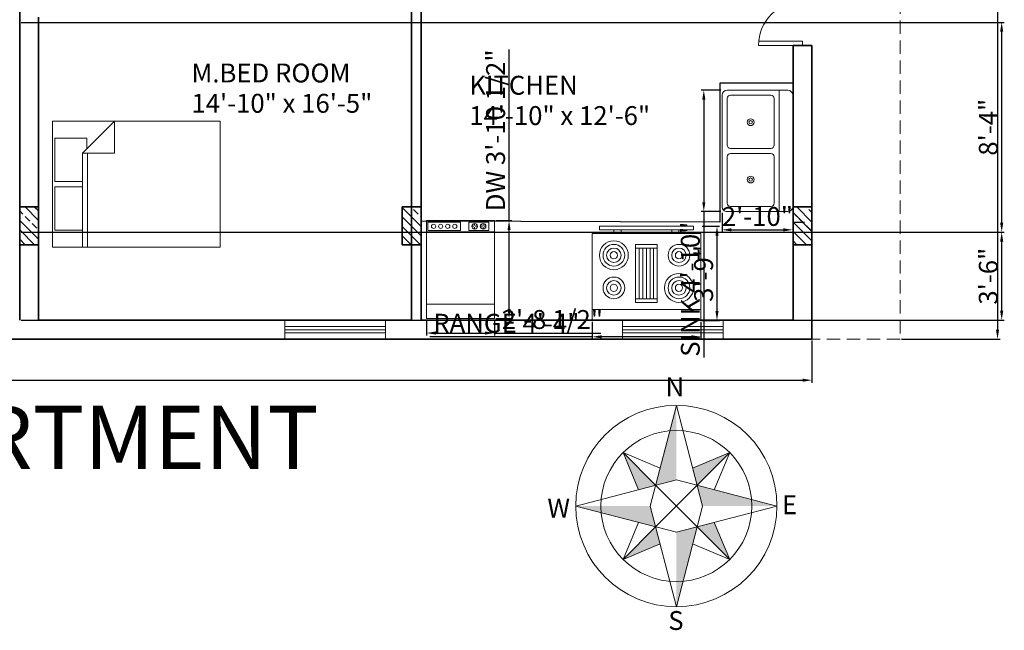
# Model space of a CAD drawing. Units: inches. Extents: x 2081 to 4786, y 1256 to 3802.
# Tile 6 of 7: x 2685 to 3155, y 1294 to 1585. Entities that reach past the tile are written whole.
import ezdxf

# ---------------------------------------------------------------- set-up
doc = ezdxf.new("R2010")
doc.units = ezdxf.units.IN
doc.linetypes.add('HIDDEN', pattern=[9.525, 6.35, -3.175])
for name, color, linetype, lineweight in [('A-ANNO-DIMS', 18, 'Continuous', 18), ('A-ANNO-SYMB', 18, 'Continuous', 18), ('A-ANNO-TITL', 18, 'Continuous', 35), ('A-AREA-IDEN', 18, 'Continuous', 18), ('A-COLS', 1, 'Continuous', 35), ('A-DOOR', 5, 'Continuous', 18), ('A-EQPM', 11, 'Continuous', 18), ('A-FLOR-CASE', 7, 'Continuous', 25), ('A-FLOR-FIXT', 18, 'Continuous', 18), ('A-FLOR-OVHD', 18, 'HIDDEN', 18), ('A-FURN', 5, 'Continuous', 18), ('A-GLAZ', 11, 'Continuous', 18), ('A-WALL', 7, 'Continuous', 35)]:
    doc.layers.add(name, color=color, linetype=linetype, lineweight=lineweight)
doc.styles.get("Standard").update_dxf_attribs({"font": 'arial.ttf'})
doc.dimstyles.new('ISO-25', dxfattribs={"dimtxt": 9, "dimasz": 4.5, "dimexe": 1.25, "dimexo": 0.625, "dimtad": 1, "dimdec": 0, "dimlunit": 3, "dimtxsty": 'Standard', "dimcen": 2.5, "dimadec": 0, "dimazin": 0, "dimtfac": 1, "dimtdec": 0, "dimtmove": 0, "dimatfit": 3, "dimfxl": 1, "dimarcsym": 0})
pattern_1 = [(135, (1916.44, -3174.735), (-13.47038, -13.47038), []), (135, (1916.44, -3170.245), (-13.47038, -13.47038), []), (135, (1916.44, -3165.755), (-13.47038, -13.47038), []), (135, (1916.44, -3161.265), (-13.47038, -13.47038), [])]

# ---------------------------------------------------------------- blocks, each defined once
blk = doc.blocks.new('Bed - Queen')
for p, q in [((0, -80.00003), (0, 0)), ((0, 0), (59.99999, 0)), ((59.99999, 0), (59.99999, -80.00003)), ((7.99999, -1.2), (28.79998, -1.2)), ((7.99999, -14.4), (7.99999, -1.2)), ((28.79998, -1.2), (28.79998, -14.4)), ((31.19999, -1.2), (51.99999, -1.2)), ((31.19999, -14.4), (31.19999, -1.2)), ((51.99999, -1.2), (51.99999, -16.4)), ((0, -14.4), (44.8, -14.4)), ((44.8, -16.8), (0, -16.8)), ((59.99999, -29.6), (44.8, -14.4)), ((44.8, -14.4), (44.8, -29.6)), ((51.99999, -16.4), (46.79936, -16.4)), ((44.8, -29.6), (59.99999, -29.6)), ((59.99999, -80.00003), (0, -80.00003))]:
    blk.add_line(p, q)
blk = doc.blocks.new('Range-Oven - 30 in top')
for p, q in [((0, -3), (30, -3)), ((12, -6), (18, -6)), ((13, -20), (13, -6)), ((14, -6), (14, -20)), ((15, -20), (15, -6)), ((16, -6), (16, -20)), ((17, -20), (17, -6)), ((18, -20), (12, -20)), ((6, -24), (6, -25)), ((8, -25), (8, -24)), ((22, -25), (22, -24)), ((24, -24), (24, -25))]:
    blk.add_line(p, q)
for points in [[(0, -24), (0, 0), (30, 0), (30, -24)], [(12, -21), (12, -5), (18, -5), (18, -21)], [(2, -26), (2, -25), (28, -25), (28, -26)]]:
    blk.add_lwpolyline(points, close=True)
for centre, radius in [((6, -9), 4), ((6, -9), 3), ((6, -9), 2), ((6, -9), 1), ((24, -9), 3), ((24, -9), 2), ((24, -9), 1), ((6, -18), 3), ((6, -18), 2), ((24, -18), 4), ((24, -18), 3), ((24, -18), 2), ((6, -18), 1), ((24, -18), 1)]:
    blk.add_circle(centre, radius)
blk = doc.blocks.new('Dishwasher')
for p, q in [((16, 32.5), (16.75, 32.5)), ((16.5, 32), (16.2942, 31.7942)), ((16.3156, 33.1843), (16.5, 33)), ((17, 32.75), (17, 33.5)), ((17, 32.25), (17, 31.5)), ((18, 32.5), (17.25, 32.5)), ((17.5, 33), (17.6938, 33.1938)), ((17.7061, 31.7939), (17.5, 32)), ((19, 32.5), (19.75, 32.5)), ((19.5, 32), (19.2942, 31.7942)), ((19.3156, 33.1843), (19.5, 33)), ((20, 32.75), (20, 33.5)), ((20, 32.25), (20, 31.5)), ((21, 32.5), (20.25, 32.5)), ((20.5, 33), (20.6938, 33.1938)), ((20.7061, 31.7939), (20.5, 32)), ((24, 30.5), (0, 30.5)), ((0, 5), (24, 5))]:
    blk.add_line(p, q)
for points in [[(0, 0), (0, 34.5), (24, 34.5), (24, 0)], [(0.5, 31), (0.5, 34), (12, 34), (12, 31)], [(15, 31), (15, 34), (22, 34), (22, 31)]]:
    blk.add_lwpolyline(points, close=True)
for centre, radius in [((2.5, 32.5), 0.75), ((5, 32.5), 0.75), ((7.5, 32.5), 0.75), ((10, 32.5), 0.75), ((17, 32.5), 1), ((20, 32.5), 1)]:
    blk.add_circle(centre, radius)
blk = doc.blocks.new('Sink-double - 36 in top')
for p, q in [((-18, -4), (18, -4)), ((-0.75, -18.5), (-0.75, -6.5)), ((0.75, -6.5), (0.75, -18.5))]:
    blk.add_line(p, q)
for points in [[(-16.5, 0), (16.5, 0)], [(-18, -19.5), (-18, -1.5)], [(18, -1.5), (18, -19.5)], [(-15.5, -5.5), (-1.75, -5.5)], [(1.75, -5.5), (15.5, -5.5)], [(-16.5, -18.5), (-16.5, -6.5)], [(16.5, -6.5), (16.5, -18.5)], [(-1.75, -19.5), (-15.5, -19.5)], [(15.5, -19.5), (1.75, -19.5)], [(16.5, -21), (-16.5, -21)]]:
    blk.add_lwpolyline(points)
for centre, radius in [((-8.5, -12.5), 1), ((8.5, -12.5), 1), ((-8.5, -12.5), 0.5), ((8.5, -12.5), 0.5)]:
    blk.add_circle(centre, radius)
for centre, radius, start, end in [((-16.5, -1.5), 1.5, 90, 180), ((16.5, -1.5), 1.5, 0, 90), ((-15.5, -6.5), 1, 90, 180), ((-1.75, -6.5), 1, 0, 90), ((1.75, -6.5), 1, 90, 180), ((15.5, -6.5), 1, 0, 90), ((-16.5, -19.5), 1.5, 180, 270), ((-15.5, -18.5), 1, 180, 270), ((-1.75, -18.5), 1, 270, 0), ((1.75, -18.5), 1, 180, 270), ((15.5, -18.5), 1, 270, 0), ((16.5, -19.5), 1.5, 270, 0)]:
    blk.add_arc(centre, radius, start, end)
blk = doc.blocks.new('*U19')
for q in [(-12.45, -24), (12.45, -24)]:
    blk.add_line((0, 24), q)
blk = doc.blocks.new('*U20')
at = {"layer": 'A-ANNO-SYMB', "color": 0, "linetype": 'ByBlock', "lineweight": -2, "transparency": 16777216}
blk.add_blockref('*U19', (2998.28, 1377.6), dxfattribs=at)
for p, rotation in [((2974.28, 1353.6), 90), ((3022.28, 1353.6), 270), ((2998.28, 1329.6), 180)]:
    blk.add_blockref('*U19', p, dxfattribs=dict(at, rotation=rotation))
blk = doc.blocks.new('*U21')
for q in [(-8.84, 1.4), (1.4, -8.84)]:
    blk.add_line((8.84, 8.84), q)
blk = doc.blocks.new('*U22')
at = {"layer": 'A-ANNO-SYMB', "color": 0, "linetype": 'ByBlock', "lineweight": -2, "transparency": 16777216}
for p, rotation in [((2981.66, 1370.22), 90.00000000000003), ((2981.66, 1336.98), 180), ((3014.89, 1336.98), 270)]:
    blk.add_blockref('*U21', p, dxfattribs=dict(at, rotation=rotation))
blk.add_blockref('*U21', (3014.89, 1370.22), dxfattribs=at)
blk = doc.blocks.new('*D24')
at = {"layer": 'A-ANNO-DIMS', "color": 0, "lineweight": -2, "transparency": 16777216}
for p, q in [((3105.61, 2023.17), (3152.75, 2023.17)), ((3151.5, 2018.67), (3151.5, 1437.67)), ((3105.61, 1433.17), (3152.75, 1433.17))]:
    blk.add_line(p, q, dxfattribs=at)
at = {"layer": 'A-ANNO-DIMS', "color": 0, "transparency": 16777216}
for points in [[(3150.75, 2018.67), (3152.25, 2018.67), (3151.5, 2023.17)], [(3150.75, 1437.67), (3152.25, 1437.67), (3151.5, 1433.17)]]:
    blk.add_solid(points, dxfattribs=at)
at = {"layer": 'Defpoints', "color": 0, "transparency": 16777216}
for p in [(3104.98, 2023.17), (3104.98, 1433.17), (3151.5, 1433.17)]:
    blk.add_point(p, dxfattribs=at)
at = {"layer": 'A-ANNO-DIMS', "color": 0, "transparency": 16777216, "insert": (3146.28, 1728.17), "char_height": 9, "attachment_point": 5, "rotation": 90}
blk.add_mtext('49\'-2"', dxfattribs=at)
blk = doc.blocks.new('*D26')
at = {"layer": 'A-ANNO-DIMS', "color": 0, "lineweight": -2, "transparency": 16777216}
for p, q in [((2202.98, 1432.55), (2202.98, 1412.32)), ((3062.98, 1432.55), (3062.98, 1412.32)), ((2207.48, 1413.57), (3058.48, 1413.57))]:
    blk.add_line(p, q, dxfattribs=at)
at = {"layer": 'A-ANNO-DIMS', "color": 0, "transparency": 16777216}
for points in [[(2207.48, 1414.32), (2207.48, 1412.82), (2202.98, 1413.57)], [(3058.48, 1414.32), (3058.48, 1412.82), (3062.98, 1413.57)]]:
    blk.add_solid(points, dxfattribs=at)
at = {"layer": 'Defpoints', "color": 0, "transparency": 16777216}
for p in [(2202.98, 1433.17), (3062.98, 1433.17), (3062.98, 1413.57)]:
    blk.add_point(p, dxfattribs=at)
at = {"layer": 'A-ANNO-DIMS', "color": 0, "transparency": 16777216, "insert": (2632.98, 1418.79), "char_height": 9, "attachment_point": 5}
blk.add_mtext('71\'-8"', dxfattribs=at)
blk = doc.blocks.new('DOOR-PAIR-42IN')
for p, q in [((0, 42), (21, 42)), ((0, 40), (21, 40)), ((21, 42), (21, 40)), ((0, 2), (21, 2)), ((21, 0), (21, 2)), ((0, 0), (21, 0))]:
    blk.add_line(p, q)
for centre, start, end in [((21, 42), 180, 270), ((21, 0), 90, 180)]:
    blk.add_arc(centre, 21, start, end)
blk = doc.blocks.new('WINDOW-48IN')
for p, q in [((0, 0), (0, 9)), ((0, 9), (4, 9)), ((48, 6), (0, 6)), ((4, 9), (48, 9)), ((48, 0), (48, 9)), ((48, 4.5), (0, 4.5)), ((48, 3), (0, 3)), ((48, 0), (0, 0))]:
    blk.add_line(p, q)
blk = doc.blocks.new('COLUMN-9X18IN')
h = blk.add_hatch()
h.set_pattern_fill('ANSI34', color=256, angle=90)
h.set_pattern_definition(pattern_1)
h.paths.add_polyline_path([(9, 18), (0, 18), (0, 0), (9, 0)])
h = blk.add_hatch()
h.set_pattern_fill('ANSI34', color=256, angle=90)
h.set_pattern_definition(pattern_1)
h.paths.add_polyline_path([(9, 18), (0, 18), (0, 0), (9, 0)])
h = blk.add_hatch()
h.set_pattern_fill('ANSI34', color=256, angle=90)
h.set_pattern_definition(pattern_1)
h.paths.add_polyline_path([(9, 18), (0, 18), (0, 0), (9, 0)])
h = blk.add_hatch()
h.set_pattern_fill('ANSI33', color=256, angle=90)
h.set_pattern_definition([(135, (1916.44, -3174.7355), (-4.490128, -4.490128), []), (135, (1916.44, -3170.2454), (-4.490128, -4.490128), [3.175, -1.5875])])
h.paths.add_polyline_path([(0, 0), (9, 0), (9, 18), (0, 18)])
for p, q in [((0, 0), (0, 18)), ((0, 18), (9, 18)), ((9, 18), (9, 0)), ((9, 0), (0, 0))]:
    blk.add_line(p, q)
blk = doc.blocks.new('*D63')
at = {"layer": 'A-ANNO-DIMS', "color": 0, "lineweight": -2, "transparency": 16777216}
for p, q in [((2958.1, 1441.42), (2958.1, 1433.03)), ((3009.89, 1441.42), (3009.89, 1433.03)), ((2958.1, 1434.28), (2880.68, 1434.28)), ((3005.39, 1434.28), (2962.6, 1434.28))]:
    blk.add_line(p, q, dxfattribs=at)
at = {"layer": 'A-ANNO-DIMS', "color": 0, "transparency": 16777216}
for points in [[(2962.6, 1435.03), (2962.6, 1433.53), (2958.1, 1434.28)], [(3005.39, 1435.03), (3005.39, 1433.53), (3009.89, 1434.28)]]:
    blk.add_solid(points, dxfattribs=at)
at = {"layer": 'Defpoints', "color": 0, "transparency": 16777216}
for p in [(2958.1, 1442.05), (3009.89, 1442.05), (2958.1, 1434.28)]:
    blk.add_point(p, dxfattribs=at)
at = {"layer": 'A-ANNO-DIMS', "color": 0, "transparency": 16777216, "insert": (2917.14, 1439.56), "char_height": 9, "attachment_point": 5}
blk.add_mtext('RANGE 4\'-4"', dxfattribs=at)
blk = doc.blocks.new('*D64')
at = {"layer": 'A-ANNO-DIMS', "color": 0, "lineweight": -2, "transparency": 16777216}
for p, q in [((3010.52, 1486.94), (3018.91, 1486.94)), ((3017.66, 1482.44), (3017.66, 1446.55)), ((3010.52, 1442.05), (3018.91, 1442.05))]:
    blk.add_line(p, q, dxfattribs=at)
at = {"layer": 'A-ANNO-DIMS', "color": 0, "transparency": 16777216}
for points in [[(3016.91, 1482.44), (3018.41, 1482.44), (3017.66, 1486.94)], [(3016.91, 1446.55), (3018.41, 1446.55), (3017.66, 1442.05)]]:
    blk.add_solid(points, dxfattribs=at)
at = {"layer": 'Defpoints', "color": 0, "transparency": 16777216}
for p in [(3009.89, 1486.94), (3009.89, 1442.05), (3017.66, 1442.05)]:
    blk.add_point(p, dxfattribs=at)
at = {"layer": 'A-ANNO-DIMS', "color": 0, "transparency": 16777216, "insert": (3012.44, 1464.49), "char_height": 9, "attachment_point": 5, "rotation": 90}
blk.add_mtext('3\'-9"', dxfattribs=at)
blk = doc.blocks.new('*D67')
at = {"layer": 'A-ANNO-DIMS', "color": 0, "lineweight": -2, "transparency": 16777216}
for p, q in [((2918.46, 1489.64), (2918.46, 1571.27)), ((2912.1, 1489.64), (2919.71, 1489.64)), ((2918.46, 1447.56), (2918.46, 1485.14)), ((2912.1, 1443.06), (2919.71, 1443.06))]:
    blk.add_line(p, q, dxfattribs=at)
at = {"layer": 'A-ANNO-DIMS', "color": 0, "transparency": 16777216}
for points in [[(2917.71, 1485.14), (2919.21, 1485.14), (2918.46, 1489.64)], [(2917.71, 1447.56), (2919.21, 1447.56), (2918.46, 1443.06)]]:
    blk.add_solid(points, dxfattribs=at)
at = {"layer": 'Defpoints', "color": 0, "transparency": 16777216}
for p in [(2911.47, 1489.64), (2918.46, 1489.64), (2911.47, 1443.06)]:
    blk.add_point(p, dxfattribs=at)
at = {"layer": 'A-ANNO-DIMS', "color": 0, "transparency": 16777216, "insert": (2913.18, 1532.7), "char_height": 9, "attachment_point": 5, "rotation": 90}
blk.add_mtext('DW 3\'-10 1/2"', dxfattribs=at)
blk = doc.blocks.new('*D68')
at = {"layer": 'A-ANNO-DIMS', "color": 0, "lineweight": -2, "transparency": 16777216}
for p, q in [((2879.07, 1442.43), (2879.07, 1434.82)), ((2911.47, 1442.43), (2911.47, 1434.82)), ((2883.57, 1436.07), (2906.97, 1436.07)), ((2911.47, 1436.07), (2962.27, 1436.07))]:
    blk.add_line(p, q, dxfattribs=at)
at = {"layer": 'A-ANNO-DIMS', "color": 0, "transparency": 16777216}
for points in [[(2883.57, 1436.82), (2883.57, 1435.32), (2879.07, 1436.07)], [(2906.97, 1436.82), (2906.97, 1435.32), (2911.47, 1436.07)]]:
    blk.add_solid(points, dxfattribs=at)
at = {"layer": 'Defpoints', "color": 0, "transparency": 16777216}
for p in [(2879.07, 1443.06), (2911.47, 1443.06), (2911.47, 1436.07)]:
    blk.add_point(p, dxfattribs=at)
at = {"layer": 'A-ANNO-DIMS', "color": 0, "transparency": 16777216, "insert": (2939.12, 1441.35), "char_height": 9, "attachment_point": 5}
blk.add_mtext('2\'-8 1/2"', dxfattribs=at)
blk = doc.blocks.new('*D71')
at = {"layer": 'A-ANNO-DIMS', "color": 0, "lineweight": -2, "transparency": 16777216}
for p, q in [((3019.43, 1551.82), (3010.12, 1551.82)), ((3011.37, 1547.32), (3011.37, 1498.44)), ((3019.43, 1493.94), (3010.12, 1493.94)), ((3011.37, 1493.94), (3011.37, 1424.48))]:
    blk.add_line(p, q, dxfattribs=at)
at = {"layer": 'A-ANNO-DIMS', "color": 0, "transparency": 16777216}
for points in [[(3010.62, 1547.32), (3012.12, 1547.32), (3011.37, 1551.82)], [(3010.62, 1498.44), (3012.12, 1498.44), (3011.37, 1493.94)]]:
    blk.add_solid(points, dxfattribs=at)
at = {"layer": 'Defpoints', "color": 0, "transparency": 16777216}
for p in [(3020.06, 1551.82), (3011.37, 1493.94), (3020.06, 1493.94)]:
    blk.add_point(p, dxfattribs=at)
at = {"layer": 'A-ANNO-DIMS', "color": 0, "transparency": 16777216, "insert": (3006.1, 1456.96), "char_height": 9, "attachment_point": 5, "rotation": 90}
blk.add_mtext('SINK 4\'-10"', dxfattribs=at)
blk = doc.blocks.new('*D72')
at = {"layer": 'A-ANNO-DIMS', "color": 0, "lineweight": -2, "transparency": 16777216}
for p, q in [((3020.06, 1493.32), (3020.06, 1484.01)), ((3053.82, 1493.32), (3053.82, 1484.01)), ((3024.56, 1485.26), (3049.32, 1485.26))]:
    blk.add_line(p, q, dxfattribs=at)
at = {"layer": 'A-ANNO-DIMS', "color": 0, "transparency": 16777216}
for points in [[(3024.56, 1486.01), (3024.56, 1484.51), (3020.06, 1485.26)], [(3049.32, 1486.01), (3049.32, 1484.51), (3053.82, 1485.26)]]:
    blk.add_solid(points, dxfattribs=at)
at = {"layer": 'Defpoints', "color": 0, "transparency": 16777216}
for p in [(3020.06, 1493.94), (3053.82, 1493.94), (3053.82, 1485.26)]:
    blk.add_point(p, dxfattribs=at)
at = {"layer": 'A-ANNO-DIMS', "color": 0, "transparency": 16777216, "insert": (3036.94, 1490.48), "char_height": 9, "attachment_point": 5}
blk.add_mtext('2\'-10"', dxfattribs=at)
blk = doc.blocks.new('*D79')
at = {"layer": 'A-ANNO-DIMS', "color": 0, "lineweight": -2, "transparency": 16777216}
for p, q in [((2685.61, 1584.17), (3154.73, 1584.17)), ((3153.48, 1488.67), (3153.48, 1579.67)), ((2685.61, 1484.17), (3154.73, 1484.17))]:
    blk.add_line(p, q, dxfattribs=at)
at = {"layer": 'A-ANNO-DIMS', "color": 0, "transparency": 16777216}
for points in [[(3152.73, 1579.67), (3154.23, 1579.67), (3153.48, 1584.17)], [(3152.73, 1488.67), (3154.23, 1488.67), (3153.48, 1484.17)]]:
    blk.add_solid(points, dxfattribs=at)
at = {"layer": 'Defpoints', "color": 0, "transparency": 16777216}
for p in [(2684.98, 1584.17), (3153.48, 1584.17), (2684.98, 1484.17)]:
    blk.add_point(p, dxfattribs=at)
at = {"layer": 'A-ANNO-DIMS', "color": 0, "transparency": 16777216, "insert": (3148.26, 1534.17), "char_height": 9, "attachment_point": 5, "rotation": 90}
blk.add_mtext('8\'-4"', dxfattribs=at)
blk = doc.blocks.new('*D80')
at = {"layer": 'A-ANNO-DIMS', "color": 0, "lineweight": -2, "transparency": 16777216}
for p, q in [((2685.61, 1484.17), (3154.73, 1484.17)), ((3153.48, 1446.67), (3153.48, 1479.67)), ((2685.61, 1442.17), (3154.73, 1442.17))]:
    blk.add_line(p, q, dxfattribs=at)
at = {"layer": 'A-ANNO-DIMS', "color": 0, "transparency": 16777216}
for points in [[(3152.73, 1479.67), (3154.23, 1479.67), (3153.48, 1484.17)], [(3152.73, 1446.67), (3154.23, 1446.67), (3153.48, 1442.17)]]:
    blk.add_solid(points, dxfattribs=at)
at = {"layer": 'Defpoints', "color": 0, "transparency": 16777216}
for p in [(2684.98, 1484.17), (3153.48, 1484.17), (2684.98, 1442.17)]:
    blk.add_point(p, dxfattribs=at)
at = {"layer": 'A-ANNO-DIMS', "color": 0, "transparency": 16777216, "insert": (3148.26, 1463.17), "char_height": 9, "attachment_point": 5, "rotation": 90}
blk.add_mtext('3\'-6"', dxfattribs=at)

msp = doc.modelspace()

# ---------------------------------------------------------------- hatches: boundary and pattern name
at = {"layer": 'A-ANNO-SYMB'}
h = msp.add_hatch(color=256, dxfattribs=at)
h.dxf.hatch_style = 1
h.paths.add_polyline_path([(2998.28, 1401.6), (2988.39, 1363.49), (2998.28, 1366.05)])
h.paths.add_polyline_path([(2985.82, 1353.6), (2950.28, 1353.6), (2988.39, 1343.71)])
h.paths.add_polyline_path([(3008.16, 1343.71), (2998.28, 1341.15), (2998.28, 1305.6)])
h.paths.add_polyline_path([(3008.16, 1363.49), (3010.73, 1353.6), (3046.28, 1353.6)])
h = msp.add_hatch(color=256, dxfattribs=at)
h.dxf.hatch_style = 1
h.paths.add_polyline_path([(3023.73, 1379.06), (3006.05, 1371.62), (3008.16, 1363.49)])
h.paths.add_polyline_path([(2972.82, 1379.06), (2980.26, 1361.38), (2988.39, 1363.49)])
h.paths.add_polyline_path([(2988.39, 1343.71), (2972.82, 1328.14), (2990.5, 1335.58)])
h.paths.add_polyline_path([(3016.29, 1345.82), (3008.16, 1343.71), (3023.73, 1328.14)])

# ---------------------------------------------------------------- linework, layer by layer
for p, q in [((2988.39, 1363.49), (2972.82, 1379.06)), ((3008.16, 1363.49), (3023.73, 1379.06)), ((2988.39, 1363.49), (3023.73, 1328.14)), ((3008.16, 1363.49), (2988.39, 1343.71)), ((2988.39, 1343.71), (2972.82, 1328.14))]:
    msp.add_line(p, q, dxfattribs=at)
for radius in [48, 36]:
    msp.add_circle((2998.28, 1353.6), radius, dxfattribs=at)
at = {"layer": 'A-FLOR-CASE'}
for p, q in [((3018.98, 1555.2), (3018.98, 1488.9)), ((3053.98, 1555.2), (3018.98, 1555.2)), ((3018.98, 1488.9), (2876.48, 1489.44)), ((3059.38, 1488.75), (3053.98, 1488.77))]:
    msp.add_line(p, q, dxfattribs=at)
at = {"layer": 'A-FLOR-OVHD'}
for p, q in [((3104.98, 2023.17), (3104.98, 1433.17)), ((3104.98, 1433.17), (3062.98, 1433.17))]:
    msp.add_line(p, q, dxfattribs=at)
at = {"layer": 'A-WALL'}
for p, q in [((2684.98, 1442.17), (2684.98, 1780.17)), ((2876.48, 1442.17), (2876.48, 1644.17)), ((2871.98, 1442.17), (2871.98, 1639.17)), ((2693.98, 1442.17), (2693.98, 1586.67)), ((3053.98, 1573.17), (3062.98, 1573.17)), ((3053.98, 1573.17), (3053.98, 1442.17)), ((3062.98, 1573.17), (3062.98, 1433.17)), ((2871.98, 1442.17), (2693.98, 1442.17)), ((3053.98, 1442.17), (2876.48, 1442.17)), ((3062.98, 1433.17), (2202.98, 1433.17))]:
    msp.add_line(p, q, dxfattribs=at)

# ---------------------------------------------------------------- block references
at = {"layer": 'A-ANNO-SYMB'}
for name in ['*U20', '*U22']:
    msp.add_blockref(name, (0, 0), dxfattribs=at)
at = {"layer": 'A-COLS'}
for p in [(2684.98, 1478.17), (2867.48, 1478.17), (3053.98, 1478.17)]:
    msp.add_blockref('COLUMN-9X18IN', p, dxfattribs=at)
at = {"layer": 'A-DOOR'}
msp.add_blockref('DOOR-PAIR-42IN', (3037.48, 1573.17), dxfattribs=at)
at = {"layer": 'A-EQPM', "xscale": 1.350110820245621, "yscale": 1.350110820245621, "zscale": 1.350110820245621}
msp.add_blockref('Dishwasher', (2879.07, 1443.06), dxfattribs=at)
at = {"layer": 'A-EQPM', "xscale": 1.726528565405313, "yscale": 1.726528565405313, "zscale": 1.726528565405313, "rotation": 180}
msp.add_blockref('Range-Oven - 30 in top', (3009.89, 1442.05), dxfattribs=at)
at = {"layer": 'A-FLOR-FIXT', "xscale": 1.607703411851546, "yscale": 1.607703411851546, "zscale": 1.607703411851546, "rotation": 269.9999999999999}
msp.add_blockref('Sink-double - 36 in top', (3053.82, 1522.88), dxfattribs=at)
at = {"layer": 'A-FURN', "rotation": 90}
msp.add_blockref('Bed - Queen', (2700.59, 1477.03), dxfattribs=at)
at = {"layer": 'A-GLAZ'}
for p in [(2811.45, 1433.17), (2972.54, 1433.17)]:
    msp.add_blockref('WINDOW-48IN', p, dxfattribs=at)

# ---------------------------------------------------------------- texts
at = {"layer": 'A-ANNO-SYMB'}
for s, p in [('N', (2993.1, 1405.89)), ('E', (3048.68, 1349.72)), ('W', (2936.74, 1348.12)), ('S', (2994.41, 1294.53))]:
    msp.add_text(s, height=9, dxfattribs=at).set_placement(p)
at = {"layer": 'A-ANNO-TITL'}
msp.add_text('RESIDENTIAL APARTMENT', height=30.1152, dxfattribs=at).set_placement((2327.01, 1371.26))
at = {"layer": 'A-AREA-IDEN'}
for s, p in [('M.BED ROOM', (2766.92, 1555.52)), ('KITCHEN', (2899.46, 1549.68)), ('14\'-10" x 16\'-5"', (2766.92, 1541.07)), ('14\'-10" x 12\'-6"', (2899.46, 1535.22))]:
    msp.add_text(s, height=9, dxfattribs=at).set_placement(p)

# ---------------------------------------------------------------- dimensions: what is measured, and where the dimension line sits
at = {"layer": 'A-ANNO-DIMS'}
for base, p1, p2, angle, override, picture, middle in [((3151.5, 1433.17), (3104.98, 2023.17), (3104.98, 1433.17), 90, {"dimclrd": 0, "dimclre": 0, "dimclrt": 0}, '*D24', (3146.28, 1728.17)), ((3153.48, 1584.17), (2684.98, 1484.17), (2684.98, 1584.17), 90, {"dimdec": 1, "dimlfac": 1, "dimrnd": 0, "dimzin": 1, "dimdsep": 46, "dimlunit": 4, "dimfrac": 2}, '*D79', (3148.26, 1534.17)), ((3017.66, 1442.05), (3009.89, 1486.94), (3009.89, 1442.05), 270, {"dimdec": 1, "dimlfac": 1, "dimrnd": 0, "dimzin": 1, "dimdsep": 46, "dimlunit": 4, "dimfrac": 2}, '*D64', (3012.44, 1464.49)), ((3153.48, 1484.17), (2684.98, 1442.17), (2684.98, 1484.17), 90, {"dimdec": 1, "dimlfac": 1, "dimrnd": 0, "dimzin": 1, "dimdsep": 46, "dimlunit": 4, "dimfrac": 2}, '*D80', (3148.26, 1463.17))]:
    dim = msp.add_linear_dim(base=base, p1=p1, p2=p2, angle=angle, dimstyle='ISO-25', override=override, dxfattribs=at)
    dim.commit()
    dim.dimension.update_dxf_attribs({"geometry": picture, "text_midpoint": middle})
for base, p1, p2, angle, text, picture, middle in [((2918.46, 1489.64), (2911.47, 1443.06), (2911.47, 1489.64), 90, 'DW <>', '*D67', (2913.18, 1532.7)), ((3011.37, 1493.94), (3020.06, 1551.82), (3020.06, 1493.94), 270, 'SINK <>', '*D71', (3006.1, 1456.96)), ((2958.1, 1434.28), (3009.89, 1442.05), (2958.1, 1442.05), 180, 'RANGE <>', '*D63', (2917.14, 1439.56))]:
    dim = msp.add_linear_dim(base=base, p1=p1, p2=p2, angle=angle, text=text, dimstyle='ISO-25', override={"dimdec": 1, "dimlfac": 1, "dimrnd": 0, "dimzin": 1, "dimdsep": 46, "dimlunit": 4, "dimfrac": 2}, dxfattribs=at)
    dim.commit()
    dim.dimension.update_dxf_attribs({"geometry": picture, "text_midpoint": middle})
for base, p1, p2, override, picture, middle in [((3053.82, 1485.26), (3020.06, 1493.94), (3053.82, 1493.94), {"dimdec": 1, "dimlfac": 1, "dimrnd": 0, "dimzin": 1, "dimdsep": 46, "dimlunit": 4, "dimfrac": 2}, '*D72', (3036.94, 1490.48)), ((2911.47, 1436.07), (2879.07, 1443.06), (2911.47, 1443.06), {"dimdec": 1, "dimlfac": 1, "dimrnd": 0, "dimzin": 1, "dimdsep": 46, "dimlunit": 4, "dimfrac": 2}, '*D68', (2939.12, 1441.35)), ((3062.98, 1413.57), (2202.98, 1433.17), (3062.98, 1433.17), {"dimclrd": 0, "dimclre": 0, "dimclrt": 0}, '*D26', (2632.98, 1418.79))]:
    dim = msp.add_linear_dim(base=base, p1=p1, p2=p2, dimstyle='ISO-25', override=override, dxfattribs=at)
    dim.commit()
    dim.dimension.update_dxf_attribs({"geometry": picture, "text_midpoint": middle})

doc.saveas('drawing.dxf')
